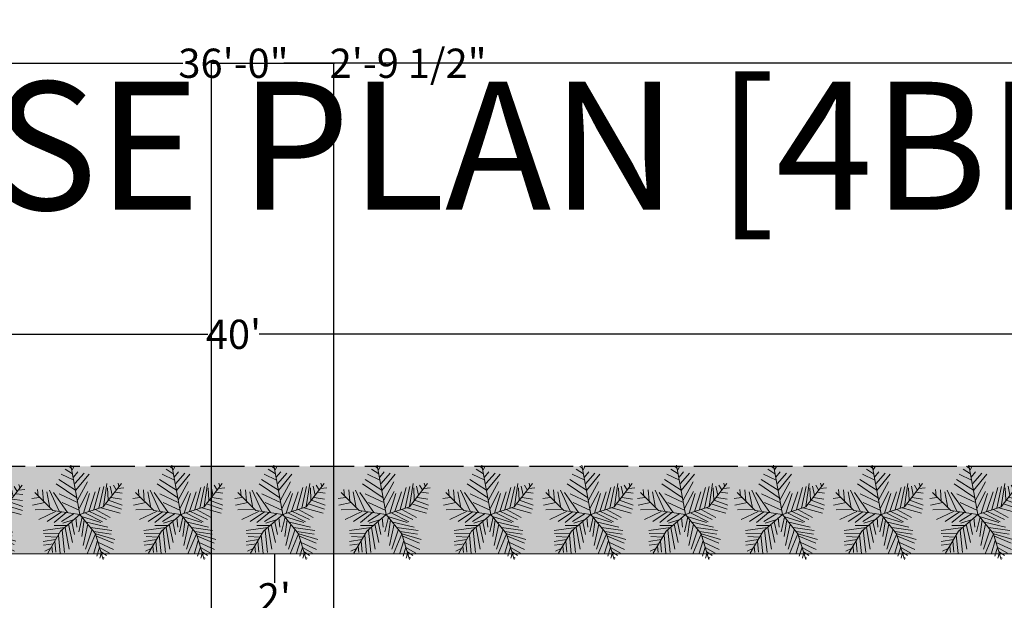
# Model space of a CAD drawing. Units: inches. Extents: x 853 to 1550, y 485 to 1596.
# Tile 17 of 18: x 1139 to 1409, y 1437 to 1596. Entities that reach past the tile are written whole.
import ezdxf

# ---------------------------------------------------------------- set-up
doc = ezdxf.new("R2010")
doc.units = ezdxf.units.IN
doc.header["$MEASUREMENT"] = 0
doc.linetypes.add('ACAD_ISO02W100', pattern=[15, 12, -3])
for name, color, linetype, lineweight in [('A-ANNO-DIMS', 2, 'Continuous', 18), ('A-ANNO-TEXT', 250, 'Continuous', 25), ('C-PROP', 8, 'ACAD_ISO02W100', 25), ('L-PLNT-TREE', 106, 'Continuous', 13), ('lawn', 106, 'Continuous', 18)]:
    doc.layers.add(name, color=color, linetype=linetype, lineweight=lineweight)
doc.layers.add('L-PLNT-PATT', color=85, linetype='Continuous', lineweight=13, true_color=0x58ba48)
doc.styles.get("Standard").update_dxf_attribs({"font": 'arial.ttf'})
doc.dimstyles.get("Standard").update_dxf_attribs({"dimtxt": 8, "dimasz": 0.18, "dimexe": 0.18, "dimexo": 0.0625, "dimgap": 0.09, "dimtad": 0, "dimtih": 1, "dimtoh": 1, "dimzin": 0, "dimdsep": 46, "dimlunit": 3, "dimtxsty": 'Standard', "dimcen": 0.09, "dimadec": 0, "dimazin": 0, "dimtfac": 1, "dimtofl": 0, "dimtmove": 0, "dimatfit": 3, "dimfxl": 1, "dimtolj": 1, "dimtzin": 0, "dimarcsym": 0})

# ---------------------------------------------------------------- blocks, each defined once
blk = doc.blocks.new('*U18')
for p, q in [((-7.288, 39.707), (-21.778, 46.673)), ((-8.737, 47.138), (-17.069, 52.711)), ((-10.186, 53.64), (-13.084, 55.962)), ((0, 0), (-10.5, 57)), ((-9.099, 51.782), (-6.563, 55.962)), ((-7.65, 43.423), (-2.578, 49.46)), ((-5.839, 35.992), (4.667, 48.067)), ((-5.114, 27.632), (10.463, 46.673)), ((-3.665, 19.273), (-27.574, 35.527)), ((-5.114, 28.097), (-24.676, 40.636)), ((-2.941, 16.486), (8.652, 37.85)), ((27, 9), (48, 36)), ((27.127, 9.056), (31.112, 35.992)), ((44.153, 36.456), (45.239, 32.741)), ((-31.5, 4.5), (-52.5, 25.5)), ((-48.585, 21.131), (-49.309, 29.026)), ((-43.513, 28.561), (-42.427, 15.558)), ((-38.442, 26.239), (-34.819, 7.663)), ((-35.544, 28.097), (-24.314, 3.947)), ((-14.533, 2.09), (-30.834, 25.31)), ((-24.314, 23.917), (-2.941, 13.7)), ((-1.129, 6.734), (9.014, 26.704)), ((3.942, 1.625), (11.187, 24.381)), ((10.101, 3.483), (17.708, 26.239)), ((16.259, 5.805), (23.142, 31.348)), ((22.055, 7.198), (27.489, 32.277)), ((31.836, 30.883), (32.561, 16.486)), ((35.096, 32.741), (37.27, 22.524)), ((38.719, 34.134), (41.979, 28.561)), ((40.53, 25.775), (48.862, 24.846)), ((43.791, 29.954), (51.036, 30.883)), ((-47.498, 19.737), (-55.83, 18.344)), ((-40.615, 13.7), (-55.105, 10.913)), ((-20.691, 13.7), (-1.129, 4.876)), ((29.662, 12.307), (48.137, 6.269)), ((33.285, 16.486), (48.862, 10.913)), ((36.183, 19.737), (48.137, 17.88)), ((-33.37, 6.269), (-52.207, 5.34)), ((-28.299, 3.483), (-47.86, -5.805)), ((-21.416, 3.018), (-38.079, -8.128)), ((0, 0), (-31.5, 4.5)), ((-15.982, 2.09), (-30.11, -9.521)), ((0, 0), (-22.5, -19.5)), ((-6.563, 1.161), (-21.416, -8.128)), ((0, 0), (27, 9)), ((0, 0), (18, -22.5)), ((6.478, 1.625), (26.04, -8.592)), ((11.187, 3.483), (30.749, -5.805)), ((18.07, 5.805), (35.096, -3.483)), ((24.229, 7.663), (46.688, 1.625)), ((-6.563, -5.805), (-19.967, -9.985)), ((-13.446, -11.378), (-8.737, -32.741)), ((-9.461, -8.592), (-6.201, -23.453)), ((-4.752, -3.483), (-3.665, -14.629)), ((2.493, -3.019), (-1.491, -20.202)), ((1.769, -2.555), (24.229, -9.521)), ((5.029, -6.27), (2.131, -25.775)), ((9.014, -11.378), (3.58, -35.992)), ((7.565, -9.056), (32.198, -14.629)), ((-17.431, -15.094), (-42.789, -18.809)), ((-24.314, -21.596), (-42.427, -22.06)), ((-22.5, -19.5), (-37.5, -45)), ((-15.257, -12.772), (-30.11, -12.772)), ((-20.691, -18.345), (-17.793, -44.352)), ((-17.069, -15.094), (-12.721, -40.172)), ((14.085, -16.951), (6.478, -40.172)), ((18.07, -22.524), (8.289, -45.745)), ((12.274, -15.094), (36.907, -18.809)), ((16.259, -19.738), (36.183, -22.989)), ((18, -22.5), (27, -52.5)), ((18.433, -22.524), (40.53, -29.026)), ((-28.299, -29.026), (-42.789, -31.348)), ((-30.834, -34.135), (-42.427, -35.528)), ((-26.849, -26.24), (-40.253, -25.775)), ((-29.023, -30.884), (-27.936, -43.887)), ((-25.038, -23.918), (-22.865, -45.281)), ((20.244, -30.419), (15.897, -44.816)), ((19.157, -25.311), (38.719, -33.206)), ((21.331, -32.741), (39.081, -40.636)), ((-34.457, -39.708), (-40.978, -42.494)), ((-32.646, -36.921), (-31.921, -44.352)), ((22.78, -37.85), (19.519, -48.532)), ((22.78, -38.314), (34.372, -44.816)), ((24.591, -43.423), (30.749, -47.603)), ((24.591, -45.745), (23.142, -50.854)), ((26.764, -49.925), (28.213, -50.854))]:
    blk.add_line(p, q)
blk = doc.blocks.new('*D19')
at = {"layer": 'A-ANNO-DIMS', "color": 0, "lineweight": -2, "transparency": 16777216}
for p, q in [((1209.13, 1449.95), (1209.13, 1442.24)), ((1209.19, 1450.13), (1209.31, 1450.13)), ((1209.13, 1426.31), (1209.13, 1434.02)), ((1209.19, 1426.13), (1209.31, 1426.13))]:
    blk.add_line(p, q, dxfattribs=at)
at = {"layer": 'A-ANNO-DIMS', "color": 0, "transparency": 16777216}
for points in [[(1209.1, 1449.95), (1209.16, 1449.95), (1209.13, 1450.13)], [(1209.1, 1426.31), (1209.16, 1426.31), (1209.13, 1426.13)]]:
    blk.add_solid(points, dxfattribs=at)
at = {"layer": 'Defpoints', "color": 0, "transparency": 16777216}
for p in [(1209.13, 1450.13), (1209.13, 1426.13), (1209.13, 1426.13)]:
    blk.add_point(p, dxfattribs=at)
at = {"layer": 'A-ANNO-DIMS', "color": 0, "transparency": 16777216, "insert": (1209.13, 1438.13), "char_height": 8, "attachment_point": 5}
blk.add_mtext("\\A1;2'", dxfattribs=at)
blk = doc.blocks.new('*D22')
at = {"layer": 'A-ANNO-DIMS', "color": 0, "lineweight": -2, "transparency": 16777216}
for p, q in [((933.94, 1511.65), (933.94, 1510.09)), ((934.12, 1510.27), (1190.9, 1510.27)), ((1461.76, 1510.27), (1204.98, 1510.27)), ((1461.94, 1511.65), (1461.94, 1510.09))]:
    blk.add_line(p, q, dxfattribs=at)
at = {"layer": 'A-ANNO-DIMS', "color": 0, "transparency": 16777216}
for points in [[(934.12, 1510.3), (934.12, 1510.24), (933.94, 1510.27)], [(1461.76, 1510.3), (1461.76, 1510.24), (1461.94, 1510.27)]]:
    blk.add_solid(points, dxfattribs=at)
at = {"layer": 'Defpoints', "color": 0, "transparency": 16777216}
for p in [(933.94, 1511.71), (1461.94, 1511.71), (1461.94, 1510.27)]:
    blk.add_point(p, dxfattribs=at)
at = {"layer": 'A-ANNO-DIMS', "color": 0, "transparency": 16777216, "insert": (1197.94, 1510.27), "char_height": 8, "attachment_point": 5}
blk.add_mtext("\\A1;40'", dxfattribs=at)
blk = doc.blocks.new('*D51')
at = {"layer": 'A-ANNO-DIMS', "color": 0, "lineweight": -2, "transparency": 16777216}
for p, q in [((1215.84, 1426.19), (1215.84, 1430.62)), ((1216.02, 1430.44), (1244.42, 1430.44)), ((1244.6, 1426.19), (1244.6, 1430.62)), ((1244.6, 1430.44), (1244.78, 1430.44))]:
    blk.add_line(p, q, dxfattribs=at)
at = {"layer": 'A-ANNO-DIMS', "color": 0, "transparency": 16777216}
for points in [[(1216.02, 1430.47), (1216.02, 1430.41), (1215.84, 1430.44)], [(1244.42, 1430.47), (1244.42, 1430.41), (1244.6, 1430.44)]]:
    blk.add_solid(points, dxfattribs=at)
at = {"layer": 'Defpoints', "color": 0, "transparency": 16777216}
for p in [(1244.6, 1430.44), (1215.84, 1426.13), (1244.6, 1426.13)]:
    blk.add_point(p, dxfattribs=at)
at = {"layer": 'A-ANNO-DIMS', "color": 0, "transparency": 16777216, "insert": (1295.48, 1430.44), "char_height": 8, "attachment_point": 5}
blk.add_mtext('\\A1;WINDOW 2\'-5" TYP.', dxfattribs=at)
blk = doc.blocks.new('*D69')
at = {"layer": 'A-ANNO-DIMS', "color": 0, "lineweight": -2, "transparency": 16777216}
for p, q in [((981.94, 1426.19), (981.94, 1584.65)), ((982.12, 1584.47), (1184.11, 1584.47)), ((1413.76, 1584.47), (1211.77, 1584.47)), ((1413.94, 1426.19), (1413.94, 1584.65))]:
    blk.add_line(p, q, dxfattribs=at)
at = {"layer": 'A-ANNO-DIMS', "color": 0, "transparency": 16777216}
for points in [[(982.12, 1584.5), (982.12, 1584.44), (981.94, 1584.47)], [(1413.76, 1584.5), (1413.76, 1584.44), (1413.94, 1584.47)]]:
    blk.add_solid(points, dxfattribs=at)
at = {"layer": 'Defpoints', "color": 0, "transparency": 16777216}
for p in [(1413.94, 1584.47), (981.94, 1426.13), (1413.94, 1426.13)]:
    blk.add_point(p, dxfattribs=at)
at = {"layer": 'A-ANNO-DIMS', "color": 0, "transparency": 16777216, "insert": (1197.94, 1584.47), "char_height": 8, "attachment_point": 5}
blk.add_mtext('\\A1;36\'-0"', dxfattribs=at)
blk = doc.blocks.new('*D81')
at = {"layer": 'A-ANNO-DIMS', "color": 0, "lineweight": -2, "transparency": 16777216}
for p, q in [((1191.94, 767.69), (1191.94, 1584.65)), ((1192.12, 1584.47), (1225.27, 1584.47)), ((1225.45, 767.69), (1225.45, 1584.65)), ((1225.45, 1584.47), (1225.63, 1584.47))]:
    blk.add_line(p, q, dxfattribs=at)
at = {"layer": 'A-ANNO-DIMS', "color": 0, "transparency": 16777216}
for points in [[(1192.12, 1584.5), (1192.12, 1584.44), (1191.94, 1584.47)], [(1225.27, 1584.5), (1225.27, 1584.44), (1225.45, 1584.47)]]:
    blk.add_solid(points, dxfattribs=at)
at = {"layer": 'Defpoints', "color": 0, "transparency": 16777216}
for p in [(1225.45, 1584.47), (1191.94, 767.63), (1225.45, 767.63)]:
    blk.add_point(p, dxfattribs=at)
at = {"layer": 'A-ANNO-DIMS', "color": 0, "transparency": 16777216, "insert": (1245.74, 1584.47), "char_height": 8, "attachment_point": 5}
blk.add_mtext('\\A1;2\'-9 1/2"', dxfattribs=at)

msp = doc.modelspace()

# ---------------------------------------------------------------- hatches: boundary and pattern name
at = {"layer": 'L-PLNT-PATT'}
h = msp.add_hatch(color=256, dxfattribs=at)
h.dxf.hatch_style = 1
h.paths.add_polyline_path([(1461.937, 1474.129), (933.937, 1474.129), (933.937, 730.129), (933.937, 622.891), (941.686, 622.891), (941.686, 604.895), (957.937, 604.895), (957.937, 1450.129), (1437.937, 1450.129), (1437.937, 604.895), (1454.646, 604.895), (1454.646, 622.891), (1461.937, 622.891), (1461.937, 734.988)])

# ---------------------------------------------------------------- linework, layer by layer
at = {"layer": 'C-PROP'}
msp.add_line((933.937, 1474.129), (1461.937, 1474.129), dxfattribs=at)
at = {"layer": 'lawn'}
msp.add_line((957.937, 1450.129), (1437.937, 1450.129), dxfattribs=at)

# ---------------------------------------------------------------- block references
at = {"layer": 'L-PLNT-TREE', "xscale": 0.2357951711934384, "yscale": 0.2357951711934384, "zscale": 0.2357951711934384}
for p in [(1128.818, 1460.518), (1155.938, 1460.956), (1183.541, 1460.956), (1211.471, 1460.956), (1239.761, 1460.956), (1268.417, 1460.956), (1295.78, 1460.956), (1321.687, 1460.956), (1348.176, 1460.956), (1375.189, 1460.956), (1401.667, 1460.956)]:
    msp.add_blockref('*U18', p, dxfattribs=at)

# ---------------------------------------------------------------- texts
at = {"layer": 'A-ANNO-TEXT'}
msp.add_text('40X60 HOUSE PLAN [4BHK]', height=35.05469, dxfattribs=at).set_placement((883.136, 1544.353))

# ---------------------------------------------------------------- dimensions: what is measured, and where the dimension line sits
at = {"layer": 'A-ANNO-DIMS'}
for base, p1, p2, picture, middle in [((1225.453, 1584.468), (1191.938, 767.629), (1225.453, 767.629), '*D81', (1245.744, 1584.468)), ((1413.937, 1584.468), (981.937, 1426.129), (1413.937, 1426.129), '*D69', (1197.937, 1584.468))]:
    dim = msp.add_linear_dim(base=base, p1=p1, p2=p2, dimstyle='Standard', override={"dimdec": 1, "dimlfac": 1, "dimrnd": 0, "dimzin": 1, "dimdsep": 46, "dimlunit": 4, "dimfrac": 2}, dxfattribs=at)
    dim.commit()
    dim.dimension.update_dxf_attribs({"geometry": picture, "text_midpoint": middle})
for base, p1, p2, text, override, picture, middle in [((1461.937, 1510.271), (933.937, 1511.712), (1461.937, 1511.712), "40'", {"dimclrd": 0, "dimclre": 0, "dimclrt": 0}, '*D22', (1197.937, 1510.271)), ((1244.597, 1430.443), (1215.842, 1426.129), (1244.597, 1426.129), 'WINDOW <> TYP.', {"dimdec": 1, "dimlfac": 1, "dimrnd": 0, "dimzin": 1, "dimdsep": 46, "dimlunit": 4, "dimfrac": 2}, '*D51', (1295.484, 1430.443))]:
    dim = msp.add_linear_dim(base=base, p1=p1, p2=p2, text=text, dimstyle='Standard', override=override, dxfattribs=at)
    dim.commit()
    dim.dimension.update_dxf_attribs({"geometry": picture, "text_midpoint": middle})
dim = msp.add_linear_dim(base=(1209.126, 1426.129), p1=(1209.126, 1450.129), p2=(1209.126, 1426.129), angle=90, dimstyle='Standard', override={"dimclrd": 0, "dimclre": 0, "dimclrt": 0}, dxfattribs=at)
dim.commit()
dim.dimension.update_dxf_attribs({"geometry": '*D19', "text_midpoint": (1209.126, 1438.129)})

doc.saveas('drawing.dxf')
